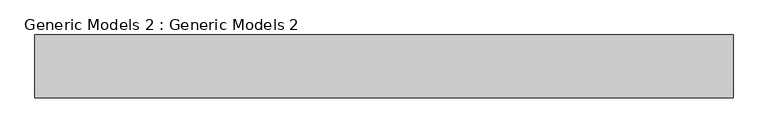
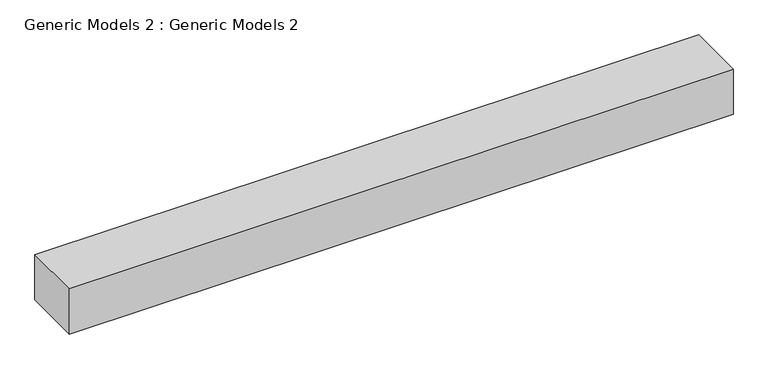
"""IFC4 building model written with IfcOpenShell, lengths in millimetres: proxy geometry, Generic Models 2 : Generic Models 2."""

from ifc_helpers import new_model, si_unit, frame, origin, place, context, project, spatial, polyline, outline, extrude, source, transform, mapped, element, save


def generic_models_2_generic_models_2_34e4dd5e(model_context):
    return source(origin(), model_context, "Body", "SweptSolid", [
        extrude(outline(polyline([(-2962.2077399, 1851.619734), (-2962.2077399, 1171.8837642), (-10506.8128458, 1171.8837642), (-10506.8128458, 1851.619734), (-2962.2077399, 1851.619734)])), frame((0.0, 0.0, 2811.1879377), z_axis=(0.0, 0.0, 1.0), x_axis=(1.0, 0.0, 0.0)), (0.0, 0.0, 1.0), 541.6120623),
    ])


if __name__ == "__main__":
    model = new_model("IFC4")
    model_context = context("Model", 3, world=origin())
    ifc_project = project(units=[si_unit("LENGTHUNIT", "METRE", prefix="MILLI")], contexts=[model_context])
    site = spatial("IfcSite", under=ifc_project)
    building = spatial("IfcBuilding", under=site)
    placement = place(None, origin())
    generic_models_2_generic_models_2_shape = generic_models_2_generic_models_2_34e4dd5e(model_context)
    element("IfcBuildingElementProxy", 1, Name="Generic Models 2 : Generic Models 2", ObjectType="Generic Models 2 : Generic Models 2", at=placement, inside=building, context=model_context, shape_type="MappedRepresentation", body=[
        mapped(generic_models_2_generic_models_2_shape, transform((0.0, 0.0, 0.0), x_axis=(1.0, 0.0, 0.0), y_axis=(0.0, 1.0, 0.0), z_axis=(0.0, 0.0, 1.0))),
    ])
    save(model, "model.ifc")
